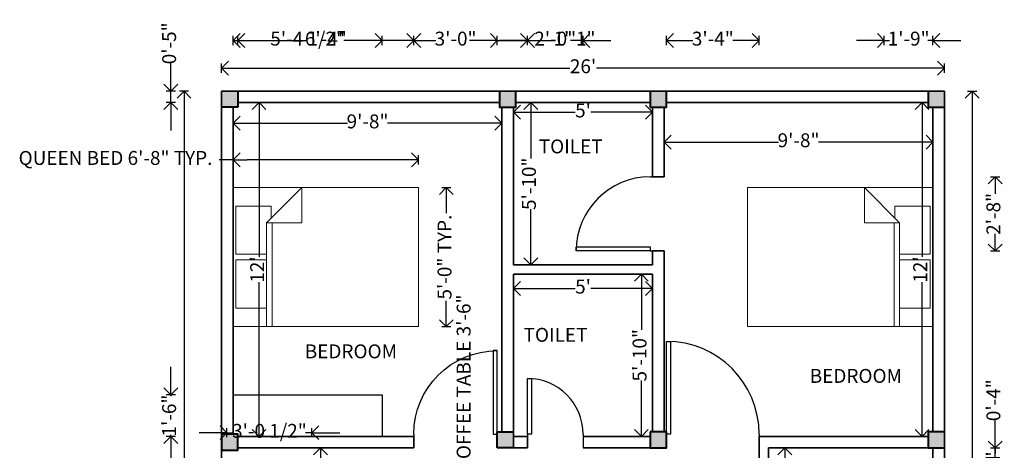
# Model space of a CAD drawing. Units: inches. Extents: x 261 to 714, y 97 to 573.
# Tile 5 of 5: x 261 to 686, y 388 to 573. Entities that reach past the tile are written whole.
import ezdxf

# ---------------------------------------------------------------- set-up
doc = ezdxf.new("R2010")
doc.units = ezdxf.units.IN
for name, color, linetype, lineweight in [('A-ANNO-DIMS', 2, 'Continuous', 18), ('A-AREA-IDEN', 7, 'Continuous', 25), ('A-COLS', 182, 'Continuous', 40), ('A-COLS-PATT', 172, 'Continuous', 13), ('A-DOOR', 182, 'Continuous', 25), ('A-FLOR-CASE', 182, 'Continuous', 25), ('A-FURN', 8, 'Continuous', 18), ('A-WALL', 182, 'Continuous', 35)]:
    doc.layers.add(name, color=color, linetype=linetype, lineweight=lineweight)
doc.styles.get("Standard").update_dxf_attribs({"font": 'arial.ttf'})
doc.dimstyles.new('ISO-25', dxfattribs={"dimtxt": 6, "dimasz": 6, "dimexe": 2, "dimexo": 2, "dimtad": 0, "dimdec": 1, "dimlunit": 3, "dimtxsty": 'Standard', "dimblk": 'OPEN90', "dimcen": 2.5, "dimclrd": 1, "dimclre": 1, "dimclrt": 1, "dimadec": 0, "dimazin": 0, "dimtfac": 1, "dimtdec": 1, "dimtmove": 0, "dimatfit": 3, "dimfxl": 2, "dimfxlon": 1, "dimarcsym": 0})

# ---------------------------------------------------------------- blocks, each defined once
blk = doc.blocks.new('*U3')
for p, q in [((0, 0), (0, -6)), ((40, 0), (40, -6))]:
    blk.add_line(p, q)
blk.add_lwpolyline([(0, 0), (0, 40), (1.75, 40), (1.75, 0)], close=True)
blk.add_arc((0, 0), 40, 0, 90)
blk = doc.blocks.new('*U4')
for p, q in [((0, 0), (0, -6)), ((36, 0), (36, -6))]:
    blk.add_line(p, q)
blk.add_lwpolyline([(0, 0), (0, 36), (1.75, 36), (1.75, 0)], close=True)
blk.add_arc((0, 0), 36, 0, 90)
blk = doc.blocks.new('*U6')
for p, q in [((0, 0), (0, -6)), ((24, 0), (24, -6))]:
    blk.add_line(p, q)
blk.add_lwpolyline([(0, 0), (0, 24), (1.75, 24), (1.75, 0)], close=True)
blk.add_arc((0, 0), 24, 0, 90)
blk = doc.blocks.new('*U5')
for p, q in [((0, 0), (0, -6)), ((32, 0), (32, -6))]:
    blk.add_line(p, q)
blk.add_lwpolyline([(0, 0), (0, 32), (1.75, 32), (1.75, 0)], close=True)
blk.add_arc((0, 0), 32, 0, 90)
blk = doc.blocks.new('_Open90')
at = {"color": 0, "linetype": 'ByBlock', "lineweight": -2}
for p, q in [((0, 0), (-1, 0)), ((-0.5, 0.5), (0, 0)), ((0, 0), (-0.5, -0.5))]:
    blk.add_line(p, q, dxfattribs=at)
blk = doc.blocks.new('*D7')
at = {"layer": 'A-ANNO-DIMS', "color": 0, "lineweight": -2, "transparency": 16777216}
for p, q in [((352.9, 530.79), (352.9, 526.79)), ((358.9, 528.79), (402.3, 528.79)), ((462.9, 528.79), (419.5, 528.79)), ((468.9, 530.79), (468.9, 526.79))]:
    blk.add_line(p, q, dxfattribs=at)
at = {"layer": 'Defpoints', "color": 0, "transparency": 16777216}
for p in [(352.9, 535.66), (468.9, 535.66), (352.9, 528.79)]:
    blk.add_point(p, dxfattribs=at)
at = {"layer": 'A-ANNO-DIMS', "color": 0, "lineweight": -2, "transparency": 16777216, "xscale": 6, "yscale": 6, "zscale": 6, "rotation": 180}
blk.add_blockref('_Open90', (352.9, 528.79), dxfattribs=at)
at = {"layer": 'A-ANNO-DIMS', "color": 0, "lineweight": -2, "transparency": 16777216, "xscale": 6, "yscale": 6, "zscale": 6}
blk.add_blockref('_Open90', (468.9, 528.79), dxfattribs=at)
at = {"layer": 'A-ANNO-DIMS', "color": 0, "transparency": 16777216, "insert": (410.9, 528.79), "char_height": 6, "attachment_point": 5}
blk.add_mtext('9\'-8"', dxfattribs=at)
blk = doc.blocks.new('*D8')
at = {"layer": 'A-ANNO-DIMS', "color": 0, "lineweight": -2, "transparency": 16777216}
for p, q in [((364.07, 537.66), (366.07, 537.66)), ((364.07, 531.66), (364.07, 471.09)), ((364.07, 399.66), (364.07, 460.22)), ((364.07, 393.66), (366.07, 393.66))]:
    blk.add_line(p, q, dxfattribs=at)
at = {"layer": 'Defpoints', "color": 0, "transparency": 16777216}
for p in [(362.2, 537.66), (362.2, 393.66), (364.07, 393.66)]:
    blk.add_point(p, dxfattribs=at)
at = {"layer": 'A-ANNO-DIMS', "color": 0, "lineweight": -2, "transparency": 16777216, "xscale": 6, "yscale": 6, "zscale": 6}
for p, rotation in [((364.07, 537.66), 90), ((364.07, 393.66), 270)]:
    blk.add_blockref('_Open90', p, dxfattribs=dict(at, rotation=rotation))
at = {"layer": 'A-ANNO-DIMS', "color": 0, "transparency": 16777216, "insert": (364.07, 465.66), "char_height": 6, "attachment_point": 5, "rotation": 90}
blk.add_mtext("12'", dxfattribs=at)
blk = doc.blocks.new('*D9')
at = {"layer": 'A-ANNO-DIMS', "color": 0, "lineweight": -2, "transparency": 16777216}
for p, q in [((473.9, 533.51), (473.9, 531.51)), ((479.9, 533.51), (500.52, 533.51)), ((527.9, 533.51), (507.29, 533.51)), ((533.9, 533.51), (533.9, 531.51))]:
    blk.add_line(p, q, dxfattribs=at)
at = {"layer": 'Defpoints', "color": 0, "transparency": 16777216}
for p in [(473.9, 534.61), (533.9, 534.61), (533.9, 533.51)]:
    blk.add_point(p, dxfattribs=at)
at = {"layer": 'A-ANNO-DIMS', "color": 0, "lineweight": -2, "transparency": 16777216, "xscale": 6, "yscale": 6, "zscale": 6, "rotation": 180}
blk.add_blockref('_Open90', (473.9, 533.51), dxfattribs=at)
at = {"layer": 'A-ANNO-DIMS', "color": 0, "lineweight": -2, "transparency": 16777216, "xscale": 6, "yscale": 6, "zscale": 6}
blk.add_blockref('_Open90', (533.9, 533.51), dxfattribs=at)
at = {"layer": 'A-ANNO-DIMS', "color": 0, "transparency": 16777216, "insert": (503.9, 533.51), "char_height": 6, "attachment_point": 5}
blk.add_mtext("5'", dxfattribs=at)
blk = doc.blocks.new('*D10')
at = {"layer": 'A-ANNO-DIMS', "color": 0, "lineweight": -2, "transparency": 16777216}
for p, q in [((481.33, 537.66), (483.33, 537.66)), ((481.33, 531.66), (481.33, 513.59)), ((481.33, 473.66), (481.33, 491.73)), ((481.33, 467.66), (483.33, 467.66))]:
    blk.add_line(p, q, dxfattribs=at)
at = {"layer": 'Defpoints', "color": 0, "transparency": 16777216}
for p in [(481.15, 537.66), (481.15, 467.66), (481.33, 467.66)]:
    blk.add_point(p, dxfattribs=at)
at = {"layer": 'A-ANNO-DIMS', "color": 0, "lineweight": -2, "transparency": 16777216, "xscale": 6, "yscale": 6, "zscale": 6}
for p, rotation in [((481.33, 537.66), 90), ((481.33, 467.66), 270)]:
    blk.add_blockref('_Open90', p, dxfattribs=dict(at, rotation=rotation))
at = {"layer": 'A-ANNO-DIMS', "color": 0, "transparency": 16777216, "insert": (481.33, 502.66), "char_height": 6, "attachment_point": 5, "rotation": 90}
blk.add_mtext('5\'-10"', dxfattribs=at)
blk = doc.blocks.new('*D11')
at = {"layer": 'A-ANNO-DIMS', "color": 0, "lineweight": -2, "transparency": 16777216}
for p, q in [((473.9, 459.51), (473.9, 455.51)), ((533.9, 459.51), (533.9, 455.51)), ((479.9, 457.51), (500.52, 457.51)), ((527.9, 457.51), (507.29, 457.51))]:
    blk.add_line(p, q, dxfattribs=at)
at = {"layer": 'Defpoints', "color": 0, "transparency": 16777216}
for p in [(473.9, 463.66), (533.9, 463.66), (533.9, 457.51)]:
    blk.add_point(p, dxfattribs=at)
at = {"layer": 'A-ANNO-DIMS', "color": 0, "lineweight": -2, "transparency": 16777216, "xscale": 6, "yscale": 6, "zscale": 6, "rotation": 180}
blk.add_blockref('_Open90', (473.9, 457.51), dxfattribs=at)
at = {"layer": 'A-ANNO-DIMS', "color": 0, "lineweight": -2, "transparency": 16777216, "xscale": 6, "yscale": 6, "zscale": 6}
blk.add_blockref('_Open90', (533.9, 457.51), dxfattribs=at)
at = {"layer": 'A-ANNO-DIMS', "color": 0, "transparency": 16777216, "insert": (503.9, 457.51), "char_height": 6, "attachment_point": 5}
blk.add_mtext("5'", dxfattribs=at)
blk = doc.blocks.new('*D12')
at = {"layer": 'A-ANNO-DIMS', "color": 0, "lineweight": -2, "transparency": 16777216}
for p, q in [((531.06, 463.66), (527.06, 463.66)), ((529.06, 457.66), (529.06, 439.59)), ((529.06, 399.66), (529.06, 417.73)), ((530.9, 393.66), (527.06, 393.66))]:
    blk.add_line(p, q, dxfattribs=at)
at = {"layer": 'Defpoints', "color": 0, "transparency": 16777216}
for p in [(533.9, 463.66), (529.06, 393.66), (532.9, 393.66)]:
    blk.add_point(p, dxfattribs=at)
at = {"layer": 'A-ANNO-DIMS', "color": 0, "lineweight": -2, "transparency": 16777216, "xscale": 6, "yscale": 6, "zscale": 6}
for p, rotation in [((529.06, 463.66), 90), ((529.06, 393.66), 270)]:
    blk.add_blockref('_Open90', p, dxfattribs=dict(at, rotation=rotation))
at = {"layer": 'A-ANNO-DIMS', "color": 0, "transparency": 16777216, "insert": (529.06, 428.66), "char_height": 6, "attachment_point": 5, "rotation": 90}
blk.add_mtext('5\'-10"', dxfattribs=at)
blk = doc.blocks.new('*D13')
at = {"layer": 'A-ANNO-DIMS', "color": 0, "lineweight": -2, "transparency": 16777216}
for p, q in [((538.9, 520.66), (538.9, 522.66)), ((654.9, 520.66), (654.9, 522.66)), ((544.9, 520.66), (588.3, 520.66)), ((648.9, 520.66), (605.5, 520.66))]:
    blk.add_line(p, q, dxfattribs=at)
at = {"layer": 'Defpoints', "color": 0, "transparency": 16777216}
for p in [(538.9, 520.66), (654.9, 520.66), (654.9, 520.66)]:
    blk.add_point(p, dxfattribs=at)
at = {"layer": 'A-ANNO-DIMS', "color": 0, "lineweight": -2, "transparency": 16777216, "xscale": 6, "yscale": 6, "zscale": 6, "rotation": 180}
blk.add_blockref('_Open90', (538.9, 520.66), dxfattribs=at)
at = {"layer": 'A-ANNO-DIMS', "color": 0, "lineweight": -2, "transparency": 16777216, "xscale": 6, "yscale": 6, "zscale": 6}
blk.add_blockref('_Open90', (654.9, 520.66), dxfattribs=at)
at = {"layer": 'A-ANNO-DIMS', "color": 0, "transparency": 16777216, "insert": (596.9, 520.66), "char_height": 6, "attachment_point": 5}
blk.add_mtext('9\'-8"', dxfattribs=at)
blk = doc.blocks.new('*D14')
at = {"layer": 'A-ANNO-DIMS', "color": 0, "lineweight": -2, "transparency": 16777216}
for p, q in [((648.18, 537.66), (652.18, 537.66)), ((650.18, 531.66), (650.18, 471.09)), ((650.18, 399.66), (650.18, 460.22)), ((648.18, 393.66), (652.18, 393.66))]:
    blk.add_line(p, q, dxfattribs=at)
at = {"layer": 'Defpoints', "color": 0, "transparency": 16777216}
for p in [(642.01, 537.66), (642.01, 393.66), (650.18, 393.66)]:
    blk.add_point(p, dxfattribs=at)
at = {"layer": 'A-ANNO-DIMS', "color": 0, "lineweight": -2, "transparency": 16777216, "xscale": 6, "yscale": 6, "zscale": 6}
for p, rotation in [((650.18, 537.66), 90), ((650.18, 393.66), 270)]:
    blk.add_blockref('_Open90', p, dxfattribs=dict(at, rotation=rotation))
at = {"layer": 'A-ANNO-DIMS', "color": 0, "transparency": 16777216, "insert": (650.18, 465.66), "char_height": 6, "attachment_point": 5, "rotation": 90}
blk.add_mtext("12'", dxfattribs=at)
blk = doc.blocks.new('*D16')
at = {"layer": 'A-ANNO-DIMS', "color": 0, "lineweight": -2, "transparency": 16777216}
for p, q in [((388.61, 388.66), (392.61, 388.66)), ((390.61, 382.66), (390.61, 344.05)), ((390.61, 298.66), (390.61, 337.27)), ((388.61, 292.66), (392.61, 292.66))]:
    blk.add_line(p, q, dxfattribs=at)
at = {"layer": 'Defpoints', "color": 0, "transparency": 16777216}
for p in [(378.75, 388.66), (378.75, 292.66), (390.61, 292.66)]:
    blk.add_point(p, dxfattribs=at)
at = {"layer": 'A-ANNO-DIMS', "color": 0, "lineweight": -2, "transparency": 16777216, "xscale": 6, "yscale": 6, "zscale": 6}
for p, rotation in [((390.61, 388.66), 90), ((390.61, 292.66), 270)]:
    blk.add_blockref('_Open90', p, dxfattribs=dict(at, rotation=rotation))
at = {"layer": 'A-ANNO-DIMS', "color": 0, "transparency": 16777216, "insert": (390.61, 340.66), "char_height": 6, "attachment_point": 5, "rotation": 90}
blk.add_mtext("8'", dxfattribs=at)
blk = doc.blocks.new('*D17')
at = {"layer": 'A-ANNO-DIMS', "color": 0, "lineweight": -2, "transparency": 16777216}
for p, q in [((593.03, 388.66), (589.03, 388.66)), ((591.03, 382.66), (591.03, 344.05)), ((591.03, 298.66), (591.03, 337.27)), ((593.03, 292.66), (589.03, 292.66))]:
    blk.add_line(p, q, dxfattribs=at)
at = {"layer": 'Defpoints', "color": 0, "transparency": 16777216}
for p in [(649.85, 388.66), (591.03, 292.66), (649.85, 292.66)]:
    blk.add_point(p, dxfattribs=at)
at = {"layer": 'A-ANNO-DIMS', "color": 0, "lineweight": -2, "transparency": 16777216, "xscale": 6, "yscale": 6, "zscale": 6}
for p, rotation in [((591.03, 388.66), 90), ((591.03, 292.66), 270)]:
    blk.add_blockref('_Open90', p, dxfattribs=dict(at, rotation=rotation))
at = {"layer": 'A-ANNO-DIMS', "color": 0, "transparency": 16777216, "insert": (591.03, 340.66), "char_height": 6, "attachment_point": 5, "rotation": 90}
blk.add_mtext("8'", dxfattribs=at)
blk = doc.blocks.new('Bed - Queen')
for p, q in [((0, -80.00003), (0, 0)), ((0, 0), (59.99999, 0)), ((59.99999, 0), (59.99999, -80.00003)), ((7.99999, -1.2), (28.79998, -1.2)), ((7.99999, -14.4), (7.99999, -1.2)), ((28.79998, -1.2), (28.79998, -14.4)), ((31.19999, -1.2), (51.99999, -1.2)), ((31.19999, -14.4), (31.19999, -1.2)), ((51.99999, -1.2), (51.99999, -16.4)), ((0, -14.4), (44.8, -14.4)), ((44.8, -16.8), (0, -16.8)), ((59.99999, -29.6), (44.8, -14.4)), ((44.8, -14.4), (44.8, -29.6)), ((51.99999, -16.4), (46.79936, -16.4)), ((44.8, -29.6), (59.99999, -29.6)), ((59.99999, -80.00003), (0, -80.00003))]:
    blk.add_line(p, q)
blk = doc.blocks.new('*D34')
at = {"layer": 'A-ANNO-DIMS', "color": 0, "lineweight": -2, "transparency": 16777216}
for p, q in [((347.9, 550.59), (347.9, 554.59)), ((353.9, 552.59), (498.14, 552.59)), ((653.9, 552.59), (509.67, 552.59)), ((659.9, 550.59), (659.9, 554.59))]:
    blk.add_line(p, q, dxfattribs=at)
at = {"layer": 'Defpoints', "color": 0, "transparency": 16777216}
for p in [(347.9, 552.59), (347.9, 542.66), (659.9, 542.66)]:
    blk.add_point(p, dxfattribs=at)
at = {"layer": 'A-ANNO-DIMS', "color": 0, "lineweight": -2, "transparency": 16777216, "xscale": 6, "yscale": 6, "zscale": 6, "rotation": 180}
blk.add_blockref('_Open90', (347.9, 552.59), dxfattribs=at)
at = {"layer": 'A-ANNO-DIMS', "color": 0, "lineweight": -2, "transparency": 16777216, "xscale": 6, "yscale": 6, "zscale": 6}
blk.add_blockref('_Open90', (659.9, 552.59), dxfattribs=at)
at = {"layer": 'A-ANNO-DIMS', "color": 0, "transparency": 16777216, "insert": (503.9, 552.59), "char_height": 6, "attachment_point": 5}
blk.add_mtext("26'", dxfattribs=at)
blk = doc.blocks.new('*D35')
at = {"layer": 'A-ANNO-DIMS', "color": 0, "lineweight": -2, "transparency": 16777216}
for p, q in [((669.78, 542.66), (673.78, 542.66)), ((671.78, 536.66), (671.78, 338.37)), ((671.78, 128.66), (671.78, 326.94)), ((669.78, 122.66), (673.78, 122.66))]:
    blk.add_line(p, q, dxfattribs=at)
at = {"layer": 'Defpoints', "color": 0, "transparency": 16777216}
for p in [(659.9, 542.66), (659.9, 122.66), (671.78, 122.66)]:
    blk.add_point(p, dxfattribs=at)
at = {"layer": 'A-ANNO-DIMS', "color": 0, "lineweight": -2, "transparency": 16777216, "xscale": 6, "yscale": 6, "zscale": 6}
for p, rotation in [((671.78, 542.66), 90), ((671.78, 122.66), 270)]:
    blk.add_blockref('_Open90', p, dxfattribs=dict(at, rotation=rotation))
at = {"layer": 'A-ANNO-DIMS', "color": 0, "transparency": 16777216, "insert": (671.78, 332.66), "char_height": 6, "attachment_point": 5, "rotation": 90}
blk.add_mtext("35'", dxfattribs=at)
blk = doc.blocks.new('*D36')
at = {"layer": 'A-ANNO-DIMS', "color": 0, "lineweight": -2, "transparency": 16777216}
for p, q in [((333.7, 542.66), (329.7, 542.66)), ((331.7, 536.66), (331.7, 338.37)), ((331.7, 128.66), (331.7, 326.94)), ((333.7, 122.66), (329.7, 122.66))]:
    blk.add_line(p, q, dxfattribs=at)
at = {"layer": 'Defpoints', "color": 0, "transparency": 16777216}
for p in [(347.9, 542.66), (331.7, 122.66), (347.9, 122.66)]:
    blk.add_point(p, dxfattribs=at)
at = {"layer": 'A-ANNO-DIMS', "color": 0, "lineweight": -2, "transparency": 16777216, "xscale": 6, "yscale": 6, "zscale": 6}
for p, rotation in [((331.7, 542.66), 90), ((331.7, 122.66), 270)]:
    blk.add_blockref('_Open90', p, dxfattribs=dict(at, rotation=rotation))
at = {"layer": 'A-ANNO-DIMS', "color": 0, "transparency": 16777216, "insert": (331.7, 332.66), "char_height": 6, "attachment_point": 5, "rotation": 90}
blk.add_mtext("35'", dxfattribs=at)
blk = doc.blocks.new('COLUMN-7IN-SQUARE')
blk.add_lwpolyline([(0, 7), (0, 2), (0, 0), (2, 0), (7, 0), (7, 2), (7, 7)], close=True)
blk = doc.blocks.new('COLUMN-7IN-TOP-EDGE')
blk.add_lwpolyline([(0, 7), (0, 2), (0, 0), (2, 0), (7, 0), (7, 2), (7, 7)])
blk = doc.blocks.new('COLUMN-7IN-SIDE-EDGE')
blk.add_lwpolyline([(7, 7), (0, 7), (0, 2), (0, 0), (2, 0), (7, 0)])
blk = doc.blocks.new('*D43')
at = {"layer": 'A-ANNO-DIMS', "color": 1, "lineweight": -2, "transparency": 16777216}
for p, q in [((352.9, 511.02), (352.9, 515.02)), ((432.9, 511.02), (432.9, 515.02)), ((352.9, 513.02), (346.9, 513.02)), ((426.9, 513.02), (358.9, 513.02))]:
    blk.add_line(p, q, dxfattribs=at)
at = {"layer": 'Defpoints', "color": 0, "transparency": 16777216}
for p in [(352.9, 513.02), (352.9, 501.02), (432.9, 501.02)]:
    blk.add_point(p, dxfattribs=at)
at = {"layer": 'A-ANNO-DIMS', "color": 1, "lineweight": -2, "transparency": 16777216, "xscale": 6, "yscale": 6, "zscale": 6, "rotation": 180}
blk.add_blockref('_Open90', (352.9, 513.02), dxfattribs=at)
at = {"layer": 'A-ANNO-DIMS', "color": 1, "lineweight": -2, "transparency": 16777216, "xscale": 6, "yscale": 6, "zscale": 6}
blk.add_blockref('_Open90', (432.9, 513.02), dxfattribs=at)
at = {"layer": 'A-ANNO-DIMS', "color": 1, "transparency": 16777216, "insert": (302.15, 513.02), "char_height": 6, "attachment_point": 5}
blk.add_mtext('QUEEN BED 6\'-8" TYP.', dxfattribs=at)
blk = doc.blocks.new('*D44')
at = {"layer": 'A-ANNO-DIMS', "color": 1, "lineweight": -2, "transparency": 16777216}
for p, q in [((442.9, 501.02), (446.9, 501.02)), ((444.9, 495.02), (444.9, 489.94)), ((444.9, 447.02), (444.9, 452.11)), ((442.9, 441.02), (446.9, 441.02))]:
    blk.add_line(p, q, dxfattribs=at)
at = {"layer": 'Defpoints', "color": 0, "transparency": 16777216}
for p in [(432.9, 501.02), (444.9, 501.02), (432.9, 441.02)]:
    blk.add_point(p, dxfattribs=at)
at = {"layer": 'A-ANNO-DIMS', "color": 1, "lineweight": -2, "transparency": 16777216, "xscale": 6, "yscale": 6, "zscale": 6}
for p, rotation in [((444.9, 501.02), 90), ((444.9, 441.02), 270)]:
    blk.add_blockref('_Open90', p, dxfattribs=dict(at, rotation=rotation))
at = {"layer": 'A-ANNO-DIMS', "color": 1, "transparency": 16777216, "insert": (444.9, 471.02), "char_height": 6, "attachment_point": 5, "rotation": 90}
blk.add_mtext('5\'-0" TYP.', dxfattribs=at)
blk = doc.blocks.new('*D46')
at = {"layer": 'A-ANNO-DIMS', "color": 1, "lineweight": -2, "transparency": 16777216}
for p, q in [((344.24, 395.26), (338.24, 395.26)), ((350.24, 393.26), (350.24, 397.26)), ((350.24, 395.26), (352.98, 395.26)), ((386.9, 395.26), (384.16, 395.26)), ((386.9, 393.26), (386.9, 397.26)), ((392.9, 395.26), (398.9, 395.26))]:
    blk.add_line(p, q, dxfattribs=at)
at = {"layer": 'Defpoints', "color": 0, "transparency": 16777216}
for p in [(350.24, 395.26), (350.24, 382.66), (386.9, 382.66)]:
    blk.add_point(p, dxfattribs=at)
at = {"layer": 'A-ANNO-DIMS', "color": 1, "lineweight": -2, "transparency": 16777216, "xscale": 6, "yscale": 6, "zscale": 6}
blk.add_blockref('_Open90', (350.24, 395.26), dxfattribs=at)
at = {"layer": 'A-ANNO-DIMS', "color": 1, "lineweight": -2, "transparency": 16777216, "xscale": 6, "yscale": 6, "zscale": 6, "rotation": 180}
blk.add_blockref('_Open90', (386.9, 395.26), dxfattribs=at)
at = {"layer": 'A-ANNO-DIMS', "color": 1, "transparency": 16777216, "insert": (368.57, 395.26), "char_height": 6, "attachment_point": 5}
blk.add_mtext('3\'-0 1/2"', dxfattribs=at)
blk = doc.blocks.new('*D47')
at = {"layer": 'A-ANNO-DIMS', "color": 1, "lineweight": -2, "transparency": 16777216}
for p, q in [((453.15, 369.61), (453.15, 375.61)), ((451.15, 369.61), (455.15, 369.61)), ((453.15, 333.6), (453.15, 363.61)), ((451.15, 327.6), (455.15, 327.6))]:
    blk.add_line(p, q, dxfattribs=at)
at = {"layer": 'Defpoints', "color": 0, "transparency": 16777216}
for p in [(446.85, 369.61), (453.15, 369.61), (446.85, 327.6)]:
    blk.add_point(p, dxfattribs=at)
at = {"layer": 'A-ANNO-DIMS', "color": 1, "lineweight": -2, "transparency": 16777216, "xscale": 6, "yscale": 6, "zscale": 6}
for p, rotation in [((453.15, 369.61), 90), ((453.15, 327.6), 270)]:
    blk.add_blockref('_Open90', p, dxfattribs=dict(at, rotation=rotation))
at = {"layer": 'A-ANNO-DIMS', "color": 1, "transparency": 16777216, "insert": (453.15, 416.77), "char_height": 6, "attachment_point": 5, "rotation": 90}
blk.add_mtext('COFFEE TABLE 3\'-6"', dxfattribs=at)
blk = doc.blocks.new('*D55')
at = {"layer": 'A-ANNO-DIMS', "color": 1, "lineweight": -2, "transparency": 16777216}
for p, q in [((354.9, 562.51), (354.9, 566.51)), ((430.9, 562.51), (430.9, 566.51)), ((360.9, 564.51), (384.29, 564.51)), ((424.9, 564.51), (401.52, 564.51))]:
    blk.add_line(p, q, dxfattribs=at)
at = {"layer": 'Defpoints', "color": 0, "transparency": 16777216}
for p in [(430.9, 564.51), (354.9, 393.66), (430.9, 393.66)]:
    blk.add_point(p, dxfattribs=at)
at = {"layer": 'A-ANNO-DIMS', "color": 1, "lineweight": -2, "transparency": 16777216, "xscale": 6, "yscale": 6, "zscale": 6, "rotation": 180}
blk.add_blockref('_Open90', (354.9, 564.51), dxfattribs=at)
at = {"layer": 'A-ANNO-DIMS', "color": 1, "lineweight": -2, "transparency": 16777216, "xscale": 6, "yscale": 6, "zscale": 6}
blk.add_blockref('_Open90', (430.9, 564.51), dxfattribs=at)
at = {"layer": 'A-ANNO-DIMS', "color": 1, "transparency": 16777216, "insert": (392.9, 564.51), "char_height": 6, "attachment_point": 5}
blk.add_mtext('6\'-4"', dxfattribs=at)
blk = doc.blocks.new('*D56')
at = {"layer": 'A-ANNO-DIMS', "color": 1, "lineweight": -2, "transparency": 16777216}
for p, q in [((430.9, 562.51), (430.9, 566.51)), ((466.9, 562.51), (466.9, 566.51)), ((436.9, 564.51), (440.31, 564.51)), ((460.9, 564.51), (457.5, 564.51))]:
    blk.add_line(p, q, dxfattribs=at)
at = {"layer": 'Defpoints', "color": 0, "transparency": 16777216}
for p in [(466.9, 564.51), (430.9, 393.66), (466.9, 392.91)]:
    blk.add_point(p, dxfattribs=at)
at = {"layer": 'A-ANNO-DIMS', "color": 1, "lineweight": -2, "transparency": 16777216, "xscale": 6, "yscale": 6, "zscale": 6, "rotation": 180}
blk.add_blockref('_Open90', (430.9, 564.51), dxfattribs=at)
at = {"layer": 'A-ANNO-DIMS', "color": 1, "lineweight": -2, "transparency": 16777216, "xscale": 6, "yscale": 6, "zscale": 6}
blk.add_blockref('_Open90', (466.9, 564.51), dxfattribs=at)
at = {"layer": 'A-ANNO-DIMS', "color": 1, "transparency": 16777216, "insert": (448.9, 564.51), "char_height": 6, "attachment_point": 5}
blk.add_mtext('3\'-0"', dxfattribs=at)
blk = doc.blocks.new('*D57')
at = {"layer": 'A-ANNO-DIMS', "color": 1, "lineweight": -2, "transparency": 16777216}
for p, q in [((466.9, 562.51), (466.9, 566.51)), ((479.9, 562.51), (479.9, 566.51)), ((460.9, 564.51), (454.9, 564.51)), ((466.9, 564.51), (479.9, 564.51)), ((485.9, 564.51), (491.9, 564.51))]:
    blk.add_line(p, q, dxfattribs=at)
at = {"layer": 'Defpoints', "color": 0, "transparency": 16777216}
for p in [(479.9, 564.51), (466.9, 392.91), (479.9, 393.66)]:
    blk.add_point(p, dxfattribs=at)
at = {"layer": 'A-ANNO-DIMS', "color": 1, "lineweight": -2, "transparency": 16777216, "xscale": 6, "yscale": 6, "zscale": 6}
blk.add_blockref('_Open90', (466.9, 564.51), dxfattribs=at)
at = {"layer": 'A-ANNO-DIMS', "color": 1, "lineweight": -2, "transparency": 16777216, "xscale": 6, "yscale": 6, "zscale": 6, "rotation": 180}
blk.add_blockref('_Open90', (479.9, 564.51), dxfattribs=at)
at = {"layer": 'A-ANNO-DIMS', "color": 1, "transparency": 16777216, "insert": (500.22, 564.51), "char_height": 6, "attachment_point": 5}
blk.add_mtext('1\'-1"', dxfattribs=at)
blk = doc.blocks.new('*D58')
at = {"layer": 'A-ANNO-DIMS', "color": 1, "lineweight": -2, "transparency": 16777216}
for p, q in [((479.9, 562.51), (479.9, 566.51)), ((503.9, 562.51), (503.9, 566.51)), ((473.9, 564.51), (467.9, 564.51)), ((479.9, 564.51), (483.25, 564.51)), ((503.9, 564.51), (500.55, 564.51)), ((509.9, 564.51), (515.9, 564.51))]:
    blk.add_line(p, q, dxfattribs=at)
at = {"layer": 'Defpoints', "color": 0, "transparency": 16777216}
for p in [(503.9, 564.51), (479.9, 393.66), (503.9, 393.66)]:
    blk.add_point(p, dxfattribs=at)
at = {"layer": 'A-ANNO-DIMS', "color": 1, "lineweight": -2, "transparency": 16777216, "xscale": 6, "yscale": 6, "zscale": 6}
blk.add_blockref('_Open90', (479.9, 564.51), dxfattribs=at)
at = {"layer": 'A-ANNO-DIMS', "color": 1, "lineweight": -2, "transparency": 16777216, "xscale": 6, "yscale": 6, "zscale": 6, "rotation": 180}
blk.add_blockref('_Open90', (503.9, 564.51), dxfattribs=at)
at = {"layer": 'A-ANNO-DIMS', "color": 1, "transparency": 16777216, "insert": (491.9, 564.51), "char_height": 6, "attachment_point": 5}
blk.add_mtext('2\'-0"', dxfattribs=at)
blk = doc.blocks.new('*D59')
at = {"layer": 'A-ANNO-DIMS', "color": 1, "lineweight": -2, "transparency": 16777216}
for p, q in [((539.9, 562.51), (539.9, 566.51)), ((579.9, 562.51), (579.9, 566.51)), ((545.9, 564.51), (551.31, 564.51)), ((573.9, 564.51), (568.5, 564.51))]:
    blk.add_line(p, q, dxfattribs=at)
at = {"layer": 'Defpoints', "color": 0, "transparency": 16777216}
for p in [(579.9, 564.51), (539.9, 392.91), (579.9, 393.66)]:
    blk.add_point(p, dxfattribs=at)
at = {"layer": 'A-ANNO-DIMS', "color": 1, "lineweight": -2, "transparency": 16777216, "xscale": 6, "yscale": 6, "zscale": 6, "rotation": 180}
blk.add_blockref('_Open90', (539.9, 564.51), dxfattribs=at)
at = {"layer": 'A-ANNO-DIMS', "color": 1, "lineweight": -2, "transparency": 16777216, "xscale": 6, "yscale": 6, "zscale": 6}
blk.add_blockref('_Open90', (579.9, 564.51), dxfattribs=at)
at = {"layer": 'A-ANNO-DIMS', "color": 1, "transparency": 16777216, "insert": (559.9, 564.51), "char_height": 6, "attachment_point": 5}
blk.add_mtext('3\'-4"', dxfattribs=at)
blk = doc.blocks.new('*D60')
at = {"layer": 'A-ANNO-DIMS', "color": 1, "lineweight": -2, "transparency": 16777216}
for p, q in [((679.75, 505.66), (683.75, 505.66)), ((681.75, 499.66), (681.75, 498.31)), ((681.75, 479.66), (681.75, 481.01)), ((679.75, 473.66), (683.75, 473.66))]:
    blk.add_line(p, q, dxfattribs=at)
at = {"layer": 'Defpoints', "color": 0, "transparency": 16777216}
for p in [(533.9, 505.66), (681.75, 505.66), (533.9, 473.66)]:
    blk.add_point(p, dxfattribs=at)
at = {"layer": 'A-ANNO-DIMS', "color": 1, "lineweight": -2, "transparency": 16777216, "xscale": 6, "yscale": 6, "zscale": 6}
for p, rotation in [((681.75, 505.66), 90), ((681.75, 473.66), 270)]:
    blk.add_blockref('_Open90', p, dxfattribs=dict(at, rotation=rotation))
at = {"layer": 'A-ANNO-DIMS', "color": 1, "transparency": 16777216, "insert": (681.75, 489.66), "char_height": 6, "attachment_point": 5, "rotation": 90}
blk.add_mtext('2\'-8"', dxfattribs=at)
blk = doc.blocks.new('*D68')
at = {"layer": 'A-ANNO-DIMS', "color": 1, "lineweight": -2, "transparency": 16777216}
for p, q in [((633.9, 562.51), (633.9, 566.51)), ((654.9, 562.51), (654.9, 566.51)), ((627.9, 564.51), (621.9, 564.51)), ((633.9, 564.51), (636.09, 564.51)), ((654.9, 564.51), (652.72, 564.51)), ((660.9, 564.51), (666.9, 564.51))]:
    blk.add_line(p, q, dxfattribs=at)
at = {"layer": 'Defpoints', "color": 0, "transparency": 16777216}
for p in [(654.9, 564.51), (654.9, 294.66), (633.9, 292.66)]:
    blk.add_point(p, dxfattribs=at)
at = {"layer": 'A-ANNO-DIMS', "color": 1, "lineweight": -2, "transparency": 16777216, "xscale": 6, "yscale": 6, "zscale": 6}
blk.add_blockref('_Open90', (633.9, 564.51), dxfattribs=at)
at = {"layer": 'A-ANNO-DIMS', "color": 1, "lineweight": -2, "transparency": 16777216, "xscale": 6, "yscale": 6, "zscale": 6, "rotation": 180}
blk.add_blockref('_Open90', (654.9, 564.51), dxfattribs=at)
at = {"layer": 'A-ANNO-DIMS', "color": 1, "transparency": 16777216, "insert": (644.4, 564.51), "char_height": 6, "attachment_point": 5}
blk.add_mtext('1\'-9"', dxfattribs=at)
blk = doc.blocks.new('*D71')
at = {"layer": 'A-ANNO-DIMS', "color": 1, "lineweight": -2, "transparency": 16777216}
for p, q in [((326.05, 548.66), (326.05, 554.66)), ((328.05, 542.66), (324.05, 542.66)), ((326.05, 537.66), (326.05, 542.66)), ((328.05, 537.66), (324.05, 537.66)), ((326.05, 531.66), (326.05, 525.66))]:
    blk.add_line(p, q, dxfattribs=at)
at = {"layer": 'Defpoints', "color": 0, "transparency": 16777216}
for p in [(326.05, 542.66), (354.9, 542.66), (354.9, 537.66)]:
    blk.add_point(p, dxfattribs=at)
at = {"layer": 'A-ANNO-DIMS', "color": 1, "lineweight": -2, "transparency": 16777216, "xscale": 6, "yscale": 6, "zscale": 6}
for p, rotation in [((326.05, 542.66), 270), ((326.05, 537.66), 90)]:
    blk.add_blockref('_Open90', p, dxfattribs=dict(at, rotation=rotation))
at = {"layer": 'A-ANNO-DIMS', "color": 1, "transparency": 16777216, "insert": (326.05, 563.26), "char_height": 6, "attachment_point": 5, "rotation": 90}
blk.add_mtext('0\'-5"', dxfattribs=at)
blk = doc.blocks.new('*D72')
at = {"layer": 'A-ANNO-DIMS', "color": 1, "lineweight": -2, "transparency": 16777216}
for p, q in [((681.75, 394.66), (681.75, 400.66)), ((679.75, 388.66), (683.75, 388.66)), ((681.75, 388.66), (681.75, 386.47)), ((681.75, 367.66), (681.75, 369.84)), ((679.75, 367.66), (683.75, 367.66)), ((681.75, 361.66), (681.75, 355.66))]:
    blk.add_line(p, q, dxfattribs=at)
at = {"layer": 'Defpoints', "color": 0, "transparency": 16777216}
for p in [(583.9, 388.66), (681.75, 388.66), (583.9, 367.66)]:
    blk.add_point(p, dxfattribs=at)
at = {"layer": 'A-ANNO-DIMS', "color": 1, "lineweight": -2, "transparency": 16777216, "xscale": 6, "yscale": 6, "zscale": 6}
for p, rotation in [((681.75, 388.66), 270), ((681.75, 367.66), 90)]:
    blk.add_blockref('_Open90', p, dxfattribs=dict(at, rotation=rotation))
at = {"layer": 'A-ANNO-DIMS', "color": 1, "transparency": 16777216, "insert": (681.75, 378.16), "char_height": 6, "attachment_point": 5, "rotation": 90}
blk.add_mtext('1\'-9"', dxfattribs=at)
blk = doc.blocks.new('*D73')
at = {"layer": 'A-ANNO-DIMS', "color": 1, "lineweight": -2, "transparency": 16777216}
for p, q in [((352.9, 562.51), (352.9, 566.51)), ((417.18, 562.51), (417.18, 566.51)), ((358.9, 564.51), (369.45, 564.51)), ((411.18, 564.51), (400.63, 564.51))]:
    blk.add_line(p, q, dxfattribs=at)
at = {"layer": 'Defpoints', "color": 0, "transparency": 16777216}
for p in [(417.18, 564.51), (352.9, 411.65), (417.18, 411.65)]:
    blk.add_point(p, dxfattribs=at)
at = {"layer": 'A-ANNO-DIMS', "color": 1, "lineweight": -2, "transparency": 16777216, "xscale": 6, "yscale": 6, "zscale": 6, "rotation": 180}
blk.add_blockref('_Open90', (352.9, 564.51), dxfattribs=at)
at = {"layer": 'A-ANNO-DIMS', "color": 1, "lineweight": -2, "transparency": 16777216, "xscale": 6, "yscale": 6, "zscale": 6}
blk.add_blockref('_Open90', (417.18, 564.51), dxfattribs=at)
at = {"layer": 'A-ANNO-DIMS', "color": 1, "transparency": 16777216, "insert": (385.04, 564.51), "char_height": 6, "attachment_point": 5}
blk.add_mtext('5\'-4 1/2"', dxfattribs=at)
blk = doc.blocks.new('*D74')
at = {"layer": 'A-ANNO-DIMS', "color": 1, "lineweight": -2, "transparency": 16777216}
for p, q in [((326.05, 417.65), (326.05, 423.65)), ((328.05, 411.65), (324.05, 411.65)), ((326.05, 411.65), (326.05, 410.97)), ((328.05, 393.66), (324.05, 393.66)), ((326.05, 393.66), (326.05, 394.34)), ((326.05, 387.66), (326.05, 381.66))]:
    blk.add_line(p, q, dxfattribs=at)
at = {"layer": 'Defpoints', "color": 0, "transparency": 16777216}
for p in [(326.05, 411.65), (417.18, 411.65), (417.18, 393.66)]:
    blk.add_point(p, dxfattribs=at)
at = {"layer": 'A-ANNO-DIMS', "color": 1, "lineweight": -2, "transparency": 16777216, "xscale": 6, "yscale": 6, "zscale": 6}
for p, rotation in [((326.05, 411.65), 270), ((326.05, 393.66), 90)]:
    blk.add_blockref('_Open90', p, dxfattribs=dict(at, rotation=rotation))
at = {"layer": 'A-ANNO-DIMS', "color": 1, "transparency": 16777216, "insert": (326.05, 402.65), "char_height": 6, "attachment_point": 5, "rotation": 90}
blk.add_mtext('1\'-6"', dxfattribs=at)
blk = doc.blocks.new('*D78')
at = {"layer": 'A-ANNO-DIMS', "color": 1, "lineweight": -2, "transparency": 16777216}
for p, q in [((681.75, 394.66), (681.75, 400.66)), ((679.75, 388.66), (683.75, 388.66)), ((681.75, 384.52), (681.75, 388.66)), ((679.75, 384.52), (683.75, 384.52)), ((681.75, 378.52), (681.75, 372.52))]:
    blk.add_line(p, q, dxfattribs=at)
at = {"layer": 'Defpoints', "color": 0, "transparency": 16777216}
for p in [(652.88, 388.66), (681.75, 388.66), (651.82, 384.52)]:
    blk.add_point(p, dxfattribs=at)
at = {"layer": 'A-ANNO-DIMS', "color": 1, "lineweight": -2, "transparency": 16777216, "xscale": 6, "yscale": 6, "zscale": 6}
for p, rotation in [((681.75, 388.66), 270), ((681.75, 384.52), 90)]:
    blk.add_blockref('_Open90', p, dxfattribs=dict(at, rotation=rotation))
at = {"layer": 'A-ANNO-DIMS', "color": 1, "transparency": 16777216, "insert": (681.75, 409.26), "char_height": 6, "attachment_point": 5, "rotation": 90}
blk.add_mtext('0\'-4"', dxfattribs=at)

msp = doc.modelspace()

# ---------------------------------------------------------------- hatches: boundary and pattern name
at = {"layer": 'A-COLS-PATT'}
h = msp.add_hatch(color=256, dxfattribs=at)
h.dxf.hatch_style = 1
h.paths.add_polyline_path([(354.9, 542.66), (347.9, 542.66), (347.9, 535.66), (354.9, 535.66)])
h.paths.add_polyline_path([(539.9, 542.66), (532.9, 542.66), (532.9, 537.66), (532.9, 535.66), (534.9, 535.66), (539.9, 535.66), (539.9, 537.66)])
h.paths.add_polyline_path([(474.9, 542.66), (467.9, 542.66), (467.9, 537.66), (467.9, 535.66), (469.9, 535.66), (474.9, 535.66), (474.9, 537.66)])
h.paths.add_polyline_path([(659.9, 542.66), (652.9, 542.66), (652.9, 537.66), (652.9, 535.66), (654.9, 535.66), (659.9, 535.66)])
h.paths.add_polyline_path([(659.9, 395.66), (652.88, 395.66), (652.88, 390.66), (652.88, 388.66), (654.88, 388.66), (659.9, 388.66)])
h.paths.add_polyline_path([(539.9, 395.66), (532.9, 395.66), (532.9, 390.66), (532.9, 388.66), (534.9, 388.66), (539.9, 388.66), (539.9, 390.66)])
h.paths.add_polyline_path([(473.9, 395.66), (466.9, 395.66), (466.9, 394.66), (466.9, 388.66), (473.9, 388.66)])
h.paths.add_polyline_path([(354.9, 394.66), (347.9, 394.66), (347.9, 389.66), (347.9, 387.66), (349.9, 387.66), (354.9, 387.66), (354.9, 389.66)])
h.paths.add_polyline_path([(540.9, 292.66), (533.9, 292.66), (533.9, 287.66), (533.9, 285.66), (535.9, 285.66), (540.9, 285.66), (540.9, 287.66)])
h.paths.add_polyline_path([(659.9, 294.66), (652.88, 294.66), (652.88, 289.66), (652.88, 287.66), (654.88, 287.66), (659.9, 287.66)])
h.paths.add_polyline_path([(473.9, 292.66), (466.9, 292.66), (466.9, 287.66), (466.9, 285.66), (468.9, 285.66), (473.9, 285.66), (473.9, 287.66)])
h.paths.add_polyline_path([(354.9, 293.66), (347.9, 293.66), (347.9, 288.66), (347.9, 286.66), (349.9, 286.66), (354.9, 286.66), (354.9, 288.66)])
h.paths.add_polyline_path([(354.9, 129.66), (347.9, 129.66), (347.9, 124.66), (347.9, 122.66), (349.9, 122.66), (354.9, 122.66), (354.9, 124.66)])
h.paths.add_polyline_path([(354.9, 168.66), (347.9, 168.66), (347.9, 163.66), (347.9, 161.66), (349.9, 161.66), (354.9, 161.66), (354.9, 163.66)])
h.paths.add_polyline_path([(473.9, 169.69), (466.95, 169.69), (466.95, 164.69), (466.95, 162.69), (468.95, 162.69), (473.9, 162.69)])
h.paths.add_polyline_path([(475.9, 129.66), (468.9, 129.66), (468.9, 124.66), (468.9, 122.66), (470.9, 122.66), (475.9, 122.66), (475.9, 124.66)])
h.paths.add_polyline_path([(540.9, 129.66), (533.9, 129.66), (533.9, 124.66), (533.9, 122.66), (535.9, 122.66), (540.9, 122.66), (540.9, 124.66)])
h.paths.add_polyline_path([(540.9, 169.66), (533.9, 169.66), (533.9, 164.66), (533.9, 162.66), (535.9, 162.66), (540.9, 162.66), (540.9, 164.66)])
h.paths.add_polyline_path([(659.9, 169.66), (652.9, 169.66), (652.9, 164.66), (652.9, 162.66), (654.9, 162.66), (659.9, 162.66)])
h.paths.add_polyline_path([(659.9, 129.66), (652.9, 129.66), (652.9, 124.66), (652.9, 122.66), (654.9, 122.66), (659.9, 122.66)])

# ---------------------------------------------------------------- linework, layer by layer
at = {"layer": 'A-COLS'}
for p, q in [((354.9, 542.66), (354.9, 535.66)), ((354.9, 535.66), (347.9, 535.66)), ((466.9, 388.66), (466.9, 395.66)), ((466.9, 395.66), (473.9, 395.66)), ((473.9, 388.66), (466.9, 388.66))]:
    msp.add_line(p, q, dxfattribs=at)
msp.add_lwpolyline([(652.9, 542.66), (652.9, 537.66), (652.9, 535.66), (654.9, 535.66), (659.9, 535.66)], dxfattribs=at)
at = {"layer": 'A-FLOR-CASE'}
for p, q in [((352.9, 411.65), (417.18, 411.65)), ((417.18, 411.65), (417.18, 393.66))]:
    msp.add_line(p, q, dxfattribs=at)
at = {"layer": 'A-WALL'}
for p, q in [((659.9, 542.66), (347.9, 542.66)), ((347.9, 542.66), (347.9, 122.66)), ((659.9, 122.66), (659.9, 542.66)), ((352.9, 535.66), (352.9, 394.66)), ((467.9, 537.66), (354.9, 537.66)), ((468.9, 535.66), (468.9, 395.66)), ((473.9, 535.66), (473.9, 467.66)), ((532.9, 537.66), (474.9, 537.66)), ((533.9, 535.66), (533.9, 505.66)), ((538.9, 535.66), (538.9, 505.66)), ((652.9, 537.66), (539.9, 537.66)), ((654.9, 395.66), (654.9, 535.66)), ((533.9, 505.66), (538.9, 505.66)), ((533.9, 473.66), (538.9, 473.66)), ((533.9, 473.66), (533.9, 467.66)), ((538.9, 473.66), (538.9, 395.66)), ((533.9, 467.66), (473.9, 467.66)), ((533.9, 463.66), (473.9, 463.66)), ((473.9, 463.66), (473.9, 388.66)), ((533.9, 463.66), (533.9, 395.66)), ((430.9, 393.66), (354.9, 393.66)), ((430.9, 388.66), (430.9, 393.66)), ((479.9, 393.66), (473.9, 393.66)), ((479.9, 388.66), (479.9, 393.66)), ((532.9, 393.66), (503.9, 393.66)), ((652.88, 393.66), (579.9, 393.66)), ((579.9, 393.66), (579.9, 328.66)), ((430.9, 388.66), (354.9, 388.66)), ((479.9, 388.66), (473.9, 388.66)), ((533.9, 388.66), (503.9, 388.66)), ((538.9, 388.66), (533.9, 388.66)), ((654.9, 388.66), (583.9, 388.66)), ((583.9, 388.66), (583.9, 328.66)), ((654.9, 294.66), (654.9, 388.66))]:
    msp.add_line(p, q, dxfattribs=at)

# ---------------------------------------------------------------- block references
at = {"layer": 'A-COLS'}
for name, p in [('COLUMN-7IN-TOP-EDGE', (467.9, 535.66)), ('COLUMN-7IN-TOP-EDGE', (532.9, 535.66)), ('COLUMN-7IN-SQUARE', (532.9, 388.66)), ('COLUMN-7IN-SIDE-EDGE', (652.88, 388.66)), ('COLUMN-7IN-SQUARE', (347.9, 387.66))]:
    msp.add_blockref(name, p, dxfattribs=at)
at = {"layer": 'A-DOOR', "rotation": 90}
msp.add_blockref('*U5', (532.9, 473.66), dxfattribs=at)
at = {"layer": 'A-DOOR'}
for name, p in [('*U3', (539.9, 394.66)), ('*U6', (479.9, 394.66))]:
    msp.add_blockref(name, p, dxfattribs=at)
at = {"layer": 'A-DOOR', "xscale": -1}
msp.add_blockref('*U4', (466.9, 394.66), dxfattribs=at)
at = {"layer": 'A-FURN', "rotation": 90}
msp.add_blockref('Bed - Queen', (352.9, 441.02), dxfattribs=at)
at = {"layer": 'A-FURN', "xscale": -1, "rotation": 270}
msp.add_blockref('Bed - Queen', (654.9, 441.02), dxfattribs=at)

# ---------------------------------------------------------------- texts
at = {"layer": 'A-AREA-IDEN', "char_height": 6, "attachment_point": 1}
for s, insert in [('{TOILET}', (484.8, 521.77)), ('{TOILET}', (478.25, 440.49)), ('{BEDROOM}', (383.82, 433.35)), ('{BEDROOM}', (601.72, 422.76))]:
    msp.add_mtext_dynamic_manual_height_columns(s, width=60.8654, gutter_width=12.5, heights=[0], dxfattribs=dict(at, insert=insert))

# ---------------------------------------------------------------- dimensions: what is measured, and where the dimension line sits
at = {"layer": 'A-ANNO-DIMS'}
for base, p1, p2, angle, override, picture, middle in [((326.05, 542.66), (354.9, 537.66), (354.9, 542.66), 90, {"dimdec": 1, "dimlfac": 1, "dimrnd": 0, "dimzin": 1, "dimdsep": 46, "dimlunit": 4, "dimfrac": 2}, '*D71', (326.05, 563.26)), ((331.7, 122.66), (347.9, 542.66), (347.9, 122.66), 90, {"dimclrd": 0, "dimclre": 0, "dimclrt": 0}, '*D36', (331.7, 332.66)), ((671.78, 122.66), (659.9, 542.66), (659.9, 122.66), 90, {"dimclrd": 0, "dimclre": 0, "dimclrt": 0}, '*D35', (671.78, 332.66)), ((364.07, 393.66), (362.2, 537.66), (362.2, 393.66), 90, {"dimclrd": 0, "dimclre": 0, "dimclrt": 0}, '*D8', (364.07, 465.66)), ((481.33, 467.66), (481.15, 537.66), (481.15, 467.66), 90, {"dimclrd": 0, "dimclre": 0, "dimclrt": 0}, '*D10', (481.33, 502.66)), ((681.75, 505.66), (533.9, 473.66), (533.9, 505.66), 90, {"dimdec": 1, "dimlfac": 1, "dimrnd": 0, "dimzin": 1, "dimdsep": 46, "dimlunit": 4, "dimfrac": 2}, '*D60', (681.75, 489.66)), ((529.06, 393.66), (533.9, 463.66), (532.9, 393.66), 90, {"dimclrd": 0, "dimclre": 0, "dimclrt": 0}, '*D12', (529.06, 428.66)), ((326.05, 411.65), (417.18, 393.66), (417.18, 411.65), 90, {"dimdec": 1, "dimlfac": 1, "dimrnd": 0, "dimzin": 1, "dimdsep": 46, "dimlunit": 4, "dimfrac": 2}, '*D74', (326.05, 402.65)), ((681.75, 388.66), (651.82, 384.52), (652.88, 388.66), 90, {"dimdec": 1, "dimlfac": 1, "dimrnd": 0, "dimzin": 1, "dimdsep": 46, "dimlunit": 4, "dimfrac": 2}, '*D78', (681.75, 409.26)), ((350.24, 395.26), (386.9, 382.66), (350.24, 382.66), 180, {"dimdec": 1, "dimlfac": 1, "dimrnd": 0, "dimzin": 1, "dimdsep": 46, "dimlunit": 4, "dimfrac": 2}, '*D46', (368.57, 395.26)), ((681.75, 388.66), (583.9, 367.66), (583.9, 388.66), 90, {"dimdec": 1, "dimlfac": 1, "dimrnd": 0, "dimzin": 1, "dimdsep": 46, "dimlunit": 4, "dimfrac": 2}, '*D72', (681.75, 378.16))]:
    dim = msp.add_linear_dim(base=base, p1=p1, p2=p2, angle=angle, dimstyle='ISO-25', override=override, dxfattribs=at)
    dim.commit()
    dim.dimension.update_dxf_attribs({"geometry": picture, "text_midpoint": middle})
for base, p1, p2, override, picture, middle in [((417.18, 564.51), (352.9, 411.65), (417.18, 411.65), {"dimdec": 1, "dimlfac": 1, "dimrnd": 0, "dimzin": 1, "dimdsep": 46, "dimlunit": 4, "dimfrac": 2}, '*D73', (385.04, 564.51)), ((430.9, 564.51), (354.9, 393.66), (430.9, 393.66), {"dimdec": 1, "dimlfac": 1, "dimrnd": 0, "dimzin": 1, "dimdsep": 46, "dimlunit": 4, "dimfrac": 2}, '*D55', (392.9, 564.51)), ((466.9, 564.51), (430.9, 393.66), (466.9, 392.91), {"dimdec": 1, "dimlfac": 1, "dimrnd": 0, "dimzin": 1, "dimdsep": 46, "dimlunit": 4, "dimfrac": 2}, '*D56', (448.9, 564.51)), ((479.9, 564.51), (466.9, 392.91), (479.9, 393.66), {"dimdec": 1, "dimlfac": 1, "dimrnd": 0, "dimzin": 1, "dimdsep": 46, "dimlunit": 4, "dimfrac": 2}, '*D57', (500.22, 564.51)), ((503.9, 564.51), (479.9, 393.66), (503.9, 393.66), {"dimdec": 1, "dimlfac": 1, "dimrnd": 0, "dimzin": 1, "dimdsep": 46, "dimlunit": 4, "dimfrac": 2}, '*D58', (491.9, 564.51)), ((579.9, 564.51), (539.9, 392.91), (579.9, 393.66), {"dimdec": 1, "dimlfac": 1, "dimrnd": 0, "dimzin": 1, "dimdsep": 46, "dimlunit": 4, "dimfrac": 2}, '*D59', (559.9, 564.51)), ((654.9, 564.51), (633.9, 292.66), (654.9, 294.66), {"dimdec": 1, "dimlfac": 1, "dimrnd": 0, "dimzin": 1, "dimdsep": 46, "dimlunit": 4, "dimfrac": 2}, '*D68', (644.4, 564.51)), ((347.9, 552.59), (659.9, 542.66), (347.9, 542.66), {"dimclrd": 0, "dimclre": 0, "dimclrt": 0}, '*D34', (503.9, 552.59)), ((352.9, 528.79), (468.9, 535.66), (352.9, 535.66), {"dimclrd": 0, "dimclre": 0, "dimclrt": 0}, '*D7', (410.9, 528.79)), ((533.9, 533.51), (473.9, 534.61), (533.9, 534.61), {"dimclrd": 0, "dimclre": 0, "dimclrt": 0}, '*D9', (503.9, 533.51)), ((654.9, 520.66), (538.9, 520.66), (654.9, 520.66), {"dimclrd": 0, "dimclre": 0, "dimclrt": 0}, '*D13', (596.9, 520.66)), ((533.9, 457.51), (473.9, 463.66), (533.9, 463.66), {"dimclrd": 0, "dimclre": 0, "dimclrt": 0}, '*D11', (503.9, 457.51))]:
    dim = msp.add_linear_dim(base=base, p1=p1, p2=p2, dimstyle='ISO-25', override=override, dxfattribs=at)
    dim.commit()
    dim.dimension.update_dxf_attribs({"geometry": picture, "text_midpoint": middle})
for base, p1, p2, picture, middle in [((650.18, 393.66), (642.01, 537.66), (642.01, 393.66), '*D14', (650.18, 465.66)), ((390.61, 292.66), (378.75, 388.66), (378.75, 292.66), '*D16', (390.61, 340.66)), ((591.03, 292.66), (649.85, 388.66), (649.85, 292.66), '*D17', (591.03, 340.66))]:
    dim = msp.add_linear_dim(base=base, p1=p1, p2=p2, angle=90, dimstyle='ISO-25', override={"dimclrd": 0, "dimclre": 0, "dimclrt": 0}, dxfattribs=at)
    dim.commit()
    dim.dimension.update_dxf_attribs({"geometry": picture, "text_midpoint": middle, "dimtype": 160})
for base, p1, p2, angle, text, picture, middle in [((352.9, 513.02), (432.9, 501.02), (352.9, 501.02), 180, 'QUEEN BED <> TYP.', '*D43', (302.15, 513.02)), ((444.9, 501.02), (432.9, 441.02), (432.9, 501.02), 90, '<> TYP.', '*D44', (444.9, 471.02)), ((453.15, 369.61), (446.85, 327.6), (446.85, 369.61), 90, 'COFFEE TABLE <>', '*D47', (453.15, 416.77))]:
    dim = msp.add_linear_dim(base=base, p1=p1, p2=p2, angle=angle, text=text, dimstyle='ISO-25', override={"dimdec": 1, "dimlfac": 1, "dimrnd": 0, "dimzin": 1, "dimdsep": 46, "dimlunit": 4, "dimfrac": 2}, dxfattribs=at)
    dim.commit()
    dim.dimension.update_dxf_attribs({"geometry": picture, "text_midpoint": middle})

doc.saveas('drawing.dxf')
